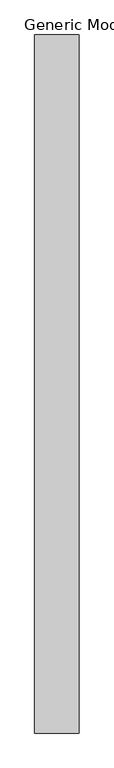
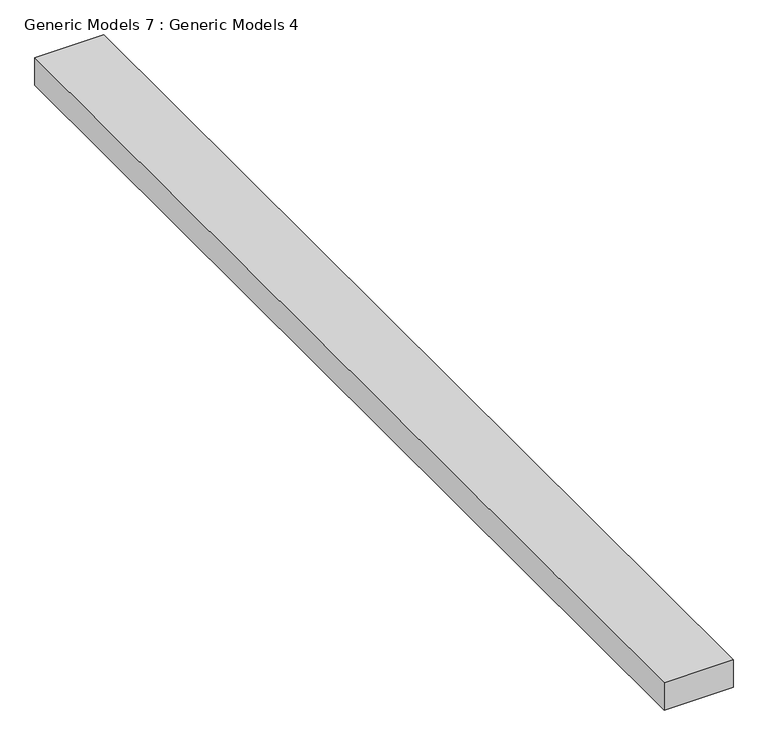
"""IFC4 building model written with IfcOpenShell, lengths in millimetres: proxy geometry, Generic Models 7 : Generic Models 4."""

from ifc_helpers import new_model, si_unit, frame, origin, place, context, project, spatial, polyline, outline, extrude, source, transform, mapped, element, save


def generic_models_7_generic_models_4_98acaeb1(model_context):
    return source(origin(), model_context, "Body", "SweptSolid", [
        extrude(outline(polyline([(14913.2564936, 13.6653678), (14913.2564936, -12716.510815), (14106.5361222, -12716.510815), (14106.5361222, 13.6653678), (14913.2564936, 13.6653678)])), frame((0.0, 0.0, 5748.0311936), z_axis=(0.0, 0.0, 1.0), x_axis=(1.0, 0.0, 0.0)), (0.0, 0.0, 1.0), 337.0869532),
    ])


if __name__ == "__main__":
    model = new_model("IFC4")
    model_context = context("Model", 3, world=origin())
    ifc_project = project(units=[si_unit("LENGTHUNIT", "METRE", prefix="MILLI")], contexts=[model_context])
    site = spatial("IfcSite", under=ifc_project)
    building = spatial("IfcBuilding", under=site)
    placement = place(None, origin())
    generic_models_7_generic_models_4_shape = generic_models_7_generic_models_4_98acaeb1(model_context)
    element("IfcBuildingElementProxy", 1, Name="Generic Models 7 : Generic Models 4", ObjectType="Generic Models 7 : Generic Models 4", at=placement, inside=building, context=model_context, shape_type="MappedRepresentation", body=[
        mapped(generic_models_7_generic_models_4_shape, transform((0.0, 0.0, 0.0), x_axis=(1.0, 0.0, 0.0), y_axis=(0.0, 1.0, 0.0), z_axis=(0.0, 0.0, 1.0))),
    ])
    save(model, "model.ifc")
